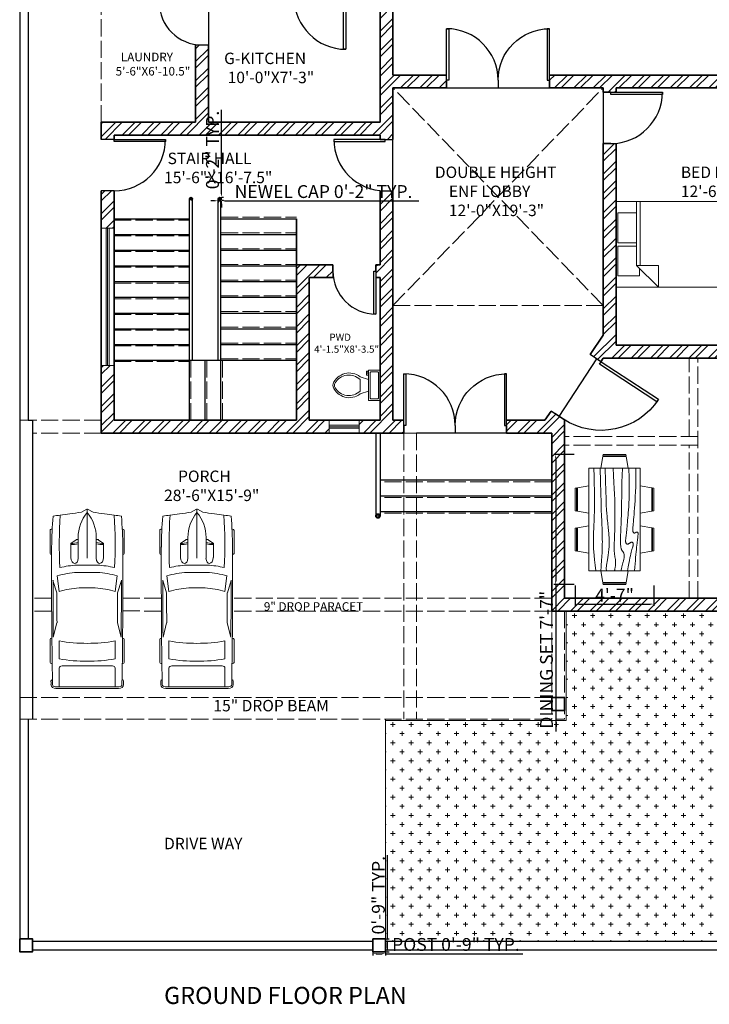
# Model space of a CAD drawing. Units: inches. Extents: x 839 to 1638, y 2998 to 4342.
# Tile 1 of 4: x 839 to 1321, y 3024 to 3713. Entities that reach past the tile are written whole.
import ezdxf

# ---------------------------------------------------------------- set-up
doc = ezdxf.new("R2010")
doc.units = ezdxf.units.IN
doc.linetypes.add('ACAD_ISO02W100', pattern=[15, 12, -3])
for name, color, linetype, lineweight in [('A-ANNO-DIMS', 2, 'Continuous', 18), ('A-ANNO-TEXT', 7, 'Continuous', 18), ('A-ANNO-TITL', 7, 'Continuous', 30), ('A-AREA-IDEN', 7, 'Continuous', 18), ('A-COLS', 7, 'Continuous', 35), ('A-DOOR', 4, 'Continuous', 25), ('A-DOOR-JAMB', 7, 'Continuous', 25), ('A-FLOR-FIXT', 9, 'Continuous', 18), ('A-FLOR-OVHD', 8, 'ACAD_ISO02W100', 18), ('A-FLOR-STRS', 7, 'Continuous', 25), ('A-FLOR-STRS-HIDN', 8, 'ACAD_ISO02W100', 13), ('A-FURN', 8, 'Continuous', 18), ('A-WALL', 7, 'Continuous', 35), ('A-WALL-OVHD', 8, 'ACAD_ISO02W100', 18), ('A-WALL-PATT', 252, 'Continuous', 13), ('C-PROP', 7, 'Continuous', 30), ('C-SITE-VEHS', 8, 'Continuous', 13), ('L-HRDS', 8, 'Continuous', 18)]:
    doc.layers.add(name, color=color, linetype=linetype, lineweight=lineweight)
doc.layers.add('A-GLAZ', color=244, linetype='Continuous', lineweight=20, true_color=0x991b1e)
doc.layers.add('L-SITE-PATT', color=116, linetype='Continuous', lineweight=13, true_color=0x136734)
doc.styles.get("Standard").update_dxf_attribs({"font": 'arial.ttf'})
doc.dimstyles.new('ISO-25', dxfattribs={"dimtxt": 9, "dimasz": 2.5, "dimexe": 1.25, "dimexo": 0.625, "dimtad": 1, "dimlunit": 3, "dimtxsty": 'Standard', "dimcen": 2.5, "dimadec": 0, "dimazin": 0, "dimtfac": 1, "dimtmove": 0, "dimatfit": 3, "dimfxl": 1, "dimarcsym": 0})

# ---------------------------------------------------------------- blocks, each defined once
blk = doc.blocks.new('*U3')
for p, q in [((-40, 0), (-40, 6)), ((0, 0), (0, 6))]:
    blk.add_line(p, q)
blk.add_lwpolyline([(0, 0), (0, -40), (-1.75, -40), (-1.75, 0)], close=True)
blk.add_arc((0, 0), 40, 180, 270)
blk = doc.blocks.new('*U2')
for p, q in [((0, 0), (0, -6)), ((40, 0), (40, -6))]:
    blk.add_line(p, q)
blk.add_lwpolyline([(0, 0), (0, 40), (1.75, 40), (1.75, 0)], close=True)
blk.add_arc((0, 0), 40, 0, 90)
blk = doc.blocks.new('*U6')
for p, q in [((0, 0), (0, -6)), ((-40, 0), (-40, -6))]:
    blk.add_line(p, q)
blk.add_lwpolyline([(0, 0), (0, 40), (-1.75, 40), (-1.75, 0)], close=True)
blk.add_arc((0, 0), 40, 90, 180)
blk = doc.blocks.new('*U7')
for p, q in [((-40, 0), (-40, 6)), ((0, 0), (0, 6))]:
    blk.add_line(p, q)
blk.add_lwpolyline([(0, 0), (0, -40), (-1.75, -40), (-1.75, 0)], close=True)
blk.add_arc((0, 0), 40, 180, 270)
blk = doc.blocks.new('*U10')
for p, q in [((0, 0), (0, 6)), ((40, 0), (40, 6))]:
    blk.add_line(p, q)
blk.add_lwpolyline([(0, 0), (0, -40), (1.75, -40), (1.75, 0)], close=True)
blk.add_arc((0, 0), 40, 270, 360)
blk = doc.blocks.new('*U11')
for p, q in [((0, 0), (0, -6)), ((-40, 0), (-40, -6))]:
    blk.add_line(p, q)
blk.add_lwpolyline([(0, 0), (0, 40), (-1.75, 40), (-1.75, 0)], close=True)
blk.add_arc((0, 0), 40, 90, 180)
blk = doc.blocks.new('*U12')
for p, q in [((-40, 0), (-40, 6)), ((0, 0), (0, 6))]:
    blk.add_line(p, q)
blk.add_lwpolyline([(0, 0), (0, -40), (-1.75, -40), (-1.75, 0)], close=True)
blk.add_arc((0, 0), 40, 180, 270)
blk = doc.blocks.new('*U15')
for p, q in [((9.5, -6), (9.5, -2)), ((-10, -8.5), (-8, -8.5)), ((-10, -9.5), (-10, -8.5)), ((-7, -9.5), (-10, -9.5)), ((-8, -8.5), (-8, -8)), ((-7, -8), (-7, -9.5)), ((-4, -8), (-6, -14)), ((4, -8), (6, -14)), ((4, -14), (-4, -14))]:
    blk.add_line(p, q)
blk.add_lwpolyline([(10.5, -8), (10.5, 0), (-10.5, 0), (-10.5, -8)], close=True)
for points in [[(-9.5, -2), (-9.5, -6)], [(8.5, -1), (-8.5, -1)], [(-8.5, -7), (8.5, -7)]]:
    blk.add_lwpolyline(points)
for centre, radius, start, end in [((-8.62, -1.88), 0.884, 81.8699, 188.1301), ((-8.62, -6.12), 0.884, 171.8699, 278.1301), ((8.62, -1.88), 0.884, 351.8699, 98.1301), ((8.62, -6.12), 0.884, 261.8699, 8.1301), ((3.52, -21.58), 12.17, 141.46911, 247.97143), ((4.2, -21.82), 11.33, 136.36773, 238.94682), ((-3.52, -21.58), 12.17, 292.02843, 38.53071), ((-4.2, -21.82), 11.33, 301.05301, 43.63209), ((0, -27.88), 4, 245.73182, 294.26817), ((0, -29), 4, 254.86053, 285.13947)]:
    blk.add_arc(centre, radius, start, end)
blk = doc.blocks.new('Bed - Queen')
for p, q in [((0, -80.00003), (0, 0)), ((0, 0), (59.99999, 0)), ((59.99999, 0), (59.99999, -80.00003)), ((7.99999, -1.2), (28.79998, -1.2)), ((7.99999, -14.4), (7.99999, -1.2)), ((28.79998, -1.2), (28.79998, -14.4)), ((31.19999, -1.2), (51.99999, -1.2)), ((31.19999, -14.4), (31.19999, -1.2)), ((51.99999, -1.2), (51.99999, -16.4)), ((0, -14.4), (44.8, -14.4)), ((44.8, -16.8), (0, -16.8)), ((59.99999, -29.6), (44.8, -14.4)), ((44.8, -14.4), (44.8, -29.6)), ((51.99999, -16.4), (46.79936, -16.4)), ((44.8, -29.6), (59.99999, -29.6)), ((59.99999, -80.00003), (0, -80.00003))]:
    blk.add_line(p, q)
blk = doc.blocks.new('Dining Set - 36 x 72 in.')
for p, q in [((-22.2343, 26.00059), (-23.4847, 17.99762)), ((-22.2304, 26), (-5.7608, 26)), ((-22, 27.5), (-22.1562, 26.50042)), ((-5.8416, 26.5), (-22.1534, 26.5)), ((-22, 27.5), (-6, 27.5)), ((-5.8437, 26.49966), (-6, 27.5)), ((-4.5152, 17.99762), (-5.7655, 25.99926)), ((5.7657, 26.00059), (4.5153, 17.99762)), ((5.7696, 26), (22.2392, 26)), ((6, 27.5), (5.8438, 26.50042)), ((22.1584, 26.5), (5.8466, 26.5)), ((6, 27.5), (22, 27.5)), ((22.1563, 26.49966), (22, 27.5)), ((23.4848, 17.99762), (22.2345, 25.99926)), ((36, 18), (-36, 18)), ((-36, 18), (-36, -18)), ((36, -18), (36, 18)), ((-45.5, 8), (-44.5004, 8.15617)), ((-45.5, 8), (-45.5, -8)), ((-44.5, -8.15843), (-44.5, 8.15338)), ((-44.0006, 8.23428), (-35.9976, 9.48474)), ((-44, 8.23041), (-44, -8.23915)), ((44.0006, 8.23428), (35.9976, 9.48474)), ((44, 8.23041), (44, -8.23915)), ((44.5, -8.15843), (44.5, 8.15338)), ((45.5, 8), (44.5005, 8.15617)), ((45.5, 8), (45.5, -8)), ((-44.4997, -8.15631), (-45.5, -8)), ((-35.9976, -9.48476), (-43.9993, -8.2345)), ((35.9976, -9.48476), (43.9993, -8.2345)), ((44.4997, -8.15631), (45.5, -8)), ((-36, -18), (36, -18)), ((-22.2343, -26.0006), (-23.4847, -17.99762)), ((-4.5152, -17.99762), (-5.7655, -25.99928)), ((5.7657, -26.0006), (4.5153, -17.99762)), ((23.4848, -17.99762), (22.2345, -25.99928)), ((-22.2304, -26), (-5.7608, -26)), ((-22, -27.5), (-22.1562, -26.50044)), ((-5.8416, -26.5), (-22.1534, -26.5)), ((-22, -27.5), (-6, -27.5)), ((-5.8437, -26.49967), (-6, -27.5)), ((5.7696, -26), (22.2392, -26)), ((6, -27.5), (5.8438, -26.50044)), ((22.1584, -26.5), (5.8466, -26.5)), ((6, -27.5), (22, -27.5)), ((22.1563, -26.49967), (22, -27.5))]:
    blk.add_line(p, q)
for points in [[(-36, 15), (-31.1772, 14.97754), (-26.8079, 14.91406), (-22.8538, 14.81543), (-19.276, 14.6875), (-16.0362, 14.53613), (-13.0957, 14.36718), (-10.4159, 14.18652), (-7.9583, 14), (-5.6904, 13.81315), (-3.6035, 13.63021), (-1.6954, 13.45508), (0.0365, 13.29166), (1.5945, 13.14388), (2.9811, 13.01562), (4.1988, 12.9108), (5.25, 12.83333), (6.1393, 12.78613), (6.8802, 12.76823), (7.4883, 12.77767), (7.9792, 12.8125), (8.3685, 12.87077), (8.6719, 12.95052), (8.9049, 13.0498), (9.0833, 13.16666), (9.2205, 13.29899), (9.3216, 13.44401), (9.3895, 13.59879), (9.4271, 13.76041), (9.4373, 13.92594), (9.4232, 14.09245), (9.3875, 14.257), (9.3333, 14.41666), (9.2638, 14.56917), (9.1836, 14.71484), (9.0975, 14.85465), (9.0104, 14.98958), (8.9272, 15.1206), (8.8529, 15.2487), (8.7922, 15.37483), (8.75, 15.5), (8.7305, 15.62467), (8.7344, 15.74739), (8.7617, 15.86621), (8.8125, 15.97916), (8.8867, 16.08431), (8.9844, 16.17968), (9.1055, 16.26334), (9.25, 16.33333), (9.4189, 16.38802), (9.6172, 16.42708), (9.8506, 16.45052), (10.125, 16.45833), (10.4463, 16.45052), (10.8203, 16.42708), (11.2529, 16.38802), (11.75, 16.33333), (12.3184, 16.26318), (12.9694, 16.17838), (13.7151, 16.07991), (14.5677, 15.96875), (15.5395, 15.84586), (16.6426, 15.71224), (17.8893, 15.56884), (19.2917, 15.41666), (20.859, 15.25667), (22.5879, 15.08984), (24.4721, 14.91715), (26.5052, 14.73958), (28.6809, 14.5581), (30.9929, 14.3737), (33.4347, 14.18733), (36, 14)], [(-36, 10), (-28.9766, 10.14274), (-23.1725, 10.20442), (-18.4241, 10.19775), (-14.5677, 10.13541), (-11.4399, 10.03011), (-8.877, 9.89453), (-6.7154, 9.74137), (-4.7917, 9.58333), (-2.9698, 9.43082), (-1.2246, 9.28515), (0.4415, 9.14534), (2.026, 9.01041), (3.5266, 8.87939), (4.9408, 8.7513), (6.266, 8.62516), (7.5, 8.5), (8.6411, 8.37549), (9.6914, 8.2539), (10.6538, 8.13818), (11.5312, 8.03125), (12.3267, 7.93603), (13.043, 7.85547), (13.6831, 7.79248), (14.25, 7.75), (14.7471, 7.7303), (15.1797, 7.73307), (15.5537, 7.75732), (15.875, 7.80208), (16.1494, 7.86637), (16.3828, 7.94922), (16.5811, 8.04964), (16.75, 8.16666), (16.8944, 8.29915), (17.0143, 8.44531), (17.1089, 8.60319), (17.1771, 8.77083), (17.218, 8.94629), (17.2305, 9.1276), (17.2137, 9.31282), (17.1667, 9.5), (17.0895, 9.6875), (16.987, 9.875), (16.8649, 10.0625), (16.7292, 10.25), (16.5856, 10.4375), (16.4401, 10.625), (16.2985, 10.8125), (16.1667, 11), (16.05, 11.18733), (15.9518, 11.3737), (15.8752, 11.5581), (15.8229, 11.73958), (15.798, 11.91715), (15.8034, 12.08984), (15.842, 12.25667), (15.9167, 12.41666), (16.0295, 12.56836), (16.1784, 12.70833), (16.3605, 12.83268), (16.5729, 12.9375), (16.8127, 13.01888), (17.0768, 13.07291), (17.3625, 13.0957), (17.6667, 13.08333), (17.9894, 13.03312), (18.3418, 12.94726), (18.7382, 12.82918), (19.1927, 12.68229), (19.7195, 12.51001), (20.3327, 12.31575), (21.0465, 12.10294), (21.875, 11.875), (22.8357, 11.63354), (23.959, 11.37304), (25.2786, 11.08618), (26.8282, 10.76562), (28.6414, 10.40405), (30.752, 9.99414), (33.1936, 9.52856), (36, 9)], [(-36, 5.5), (-30.7157, 5.3348), (-26.069, 5.20963), (-21.9946, 5.11767), (-18.4271, 5.05208), (-15.3009, 5.00602), (-12.5508, 4.97265), (-10.1112, 4.94515), (-7.9167, 4.91666), (-5.909, 4.88167), (-4.0586, 4.83984), (-2.3429, 4.79215), (-0.7396, 4.73958), (0.7739, 4.6831), (2.22, 4.6237), (3.6213, 4.56233), (5, 4.5), (6.373, 4.43782), (7.7344, 4.3776), (9.0723, 4.32129), (10.375, 4.27083), (11.6309, 4.22819), (12.8281, 4.19531), (13.9551, 4.17415), (15, 4.16666), (15.954, 4.17448), (16.819, 4.19791), (17.6001, 4.23698), (18.3021, 4.29166), (18.9299, 4.36198), (19.4883, 4.44791), (19.9823, 4.54948), (20.4167, 4.66666), (20.7969, 4.79899), (21.1302, 4.94401), (21.4245, 5.09879), (21.6875, 5.26041), (21.9271, 5.42594), (22.1511, 5.59245), (22.3672, 5.757), (22.5834, 5.91666), (22.8065, 6.06868), (23.0404, 6.21093), (23.2879, 6.34147), (23.5521, 6.45833), (23.8358, 6.55957), (24.142, 6.64323), (24.4735, 6.70735), (24.8334, 6.75), (25.2235, 6.76969), (25.642, 6.76692), (26.0858, 6.74267), (26.5521, 6.69791), (27.0379, 6.63362), (27.5404, 6.55078), (28.0565, 6.45036), (28.5834, 6.33333), (29.1242, 6.19987), (29.7071, 6.04687), (30.3661, 5.87044), (31.1354, 5.66666), (32.0493, 5.43164), (33.142, 5.16146), (34.4475, 4.85221), (36, 4.5)], [(-36, -1), (-30.7915, -0.6591), (-26.0195, -0.38216), (-21.6519, -0.16284), (-17.6563, 0.00521), (-14.0005, 0.12833), (-10.6523, 0.21289), (-7.5796, 0.26522), (-4.75, 0.29166), (-2.134, 0.29793), (0.2878, 0.28711), (2.5317, 0.26163), (4.6146, 0.22396), (6.5529, 0.17651), (8.3633, 0.12174), (10.0623, 0.06209), (11.6667, 0), (13.1899, -0.06201), (14.6341, -0.1211), (15.9982, -0.17432), (17.2813, -0.21875), (18.4823, -0.25147), (19.6003, -0.26953), (20.6343, -0.27002), (21.5834, -0.25), (22.4481, -0.20768), (23.2357, -0.14584), (23.9549, -0.06836), (24.6146, 0.02083), (25.2235, 0.11784), (25.7904, 0.21875), (26.3241, 0.31966), (26.8334, 0.41666), (27.3265, 0.50618), (27.8099, 0.58593), (28.2894, 0.65397), (28.7709, 0.70833), (29.2601, 0.74707), (29.763, 0.76823), (30.2855, 0.76985), (30.8334, 0.75), (31.4088, 0.70784), (31.9994, 0.64713), (32.589, 0.57275), (33.1615, 0.48958), (33.7008, 0.4025), (34.1908, 0.3164), (34.6153, 0.23616), (34.9584, 0.16666), (35.2099, 0.11165), (35.3848, 0.07031), (35.504, 0.04069), (35.5886, 0.02083), (35.6594, 0.00879), (35.7377, 0.0026), (35.8442, 0.00032), (36, 0)], [(-36, -6.5), (-27.1843, -6.31267), (-20.084, -6.1263), (-14.469, -5.9419), (-10.1094, -5.76042), (-6.7752, -5.58285), (-4.2363, -5.41016), (-2.2629, -5.24333), (-0.625, -5.08334), (0.8708, -4.93099), (2.2715, -4.78646), (3.5872, -4.64974), (4.8281, -4.52084), (6.0046, -4.39974), (7.127, -4.28646), (8.2053, -4.18099), (9.25, -4.08334), (10.2705, -3.99382), (11.2734, -3.91407), (12.2647, -3.84603), (13.25, -3.79167), (14.2354, -3.75293), (15.2266, -3.73177), (16.2295, -3.73015), (17.25, -3.75), (18.2912, -3.79248), (19.3451, -3.85547), (20.4009, -3.93604), (21.4479, -4.03125), (22.4754, -4.13819), (23.4727, -4.25391), (24.4289, -4.37549), (25.3334, -4.5), (26.1785, -4.62492), (26.9694, -4.74935), (27.7145, -4.87281), (28.4219, -4.99479), (29.1, -5.11483), (29.7572, -5.23242), (30.4016, -5.34709), (31.0417, -5.45834), (31.6837, -5.56437), (32.3262, -5.65821), (32.9658, -5.73153), (33.599, -5.77604), (34.2224, -5.78345), (34.8327, -5.74545), (35.4264, -5.65373), (36, -5.5)], [(-36, -10), (-26.4022, -9.81299), (-18.4675, -9.62891), (-11.9839, -9.45069), (-6.7396, -9.28125), (-2.5226, -9.12354), (0.8789, -8.98047), (3.6769, -8.85498), (6.0833, -8.75), (8.2767, -8.66765), (10.3021, -8.60677), (12.1712, -8.56543), (13.8958, -8.54167), (15.4876, -8.53353), (16.9583, -8.53907), (18.3197, -8.55632), (19.5834, -8.58334), (20.7616, -8.61841), (21.8685, -8.66081), (22.9188, -8.71004), (23.9271, -8.76563), (24.9081, -8.82707), (25.8763, -8.89388), (26.8465, -8.96558), (27.8334, -9.04167), (28.8474, -9.12118), (29.8828, -9.20117), (30.93, -9.27824), (31.9792, -9.34896), (33.0205, -9.40991), (34.0443, -9.45768), (35.0407, -9.48885), (36, -9.5)], [(-36, -14.5), (-30.0881, -14.33513), (-25.0332, -14.21224), (-20.7312, -14.12647), (-17.0781, -14.07292), (-13.97, -14.04671), (-11.3027, -14.04297), (-8.9724, -14.05681), (-6.875, -14.08334), (-4.9224, -14.11833), (-3.0905, -14.16016), (-1.3709, -14.20785), (0.2448, -14.26042), (1.7647, -14.3169), (3.1973, -14.3763), (4.5507, -14.43767), (5.8333, -14.5), (7.0554, -14.5621), (8.235, -14.62175), (9.3922, -14.67652), (10.5469, -14.72396), (11.7192, -14.76164), (12.929, -14.78711), (14.1965, -14.79794), (15.5417, -14.79167), (16.9933, -14.76424), (18.6152, -14.70508), (20.4804, -14.60197), (22.6615, -14.44271), (25.2312, -14.21509), (28.2624, -13.9069), (31.8277, -13.50594), (36, -13)]]:
    blk.add_lwpolyline(points)
blk = doc.blocks.new('*U19')
for p, q in [((21.1, 37.4), (21.1, 36.8)), ((46.6, 38.9), (22.4, 38.9)), ((47.8, 37.4), (47.8, 37.4)), ((70, 31.5), (86.4, 29.4)), ((88, 31.9), (74.8, 35.9)), ((134.3, 35.6), (119.3, 31.8)), ((135.5, 37.1), (135.5, 37.4)), ((136.7, 38.9), (160.9, 38.9)), ((162.1, 37.4), (162.1, 36.8)), ((186.5, -33.5), (186.5, 33.5)), ((188.4, -32.8), (188.4, 32.8)), ((138.4, 29.4), (157.2, 29.4)), ((164.5, 26.4), (164.5, -26.4)), ((186.5, 29.4), (167, 29.4)), ((32.1, 9.5), (32.1, 11.2)), ((32.3, 11.6), (36.1, 17.2)), ((36.1, 17.2), (50.9, 17.2)), ((58.9, -10.8), (58.9, 10.8)), ((66.6, -10.5), (66.6, 10.5)), ((186.5, -10.5), (186.5, 10.5)), ((3.3, 6.1), (0.1, 0.4)), ((29.8, 9.5), (51.7, 9.5)), ((82.7, 8.5), (82.7, -8.5)), ((0, 0), (51.7, 0)), ((0.1, -0.4), (3.3, -6.1)), ((29.8, -9.5), (51.7, -9.5)), ((32.1, -9.5), (32.1, -11.2)), ((32.3, -11.6), (36.1, -17.2)), ((36.1, -17.2), (50.9, -17.2)), ((86.4, -29.4), (70, -31.5)), ((157.2, -29.4), (138.4, -29.4)), ((167, -29.4), (186.5, -29.4)), ((21.1, -37.4), (21.1, -36.8)), ((46.6, -38.9), (22.4, -38.9)), ((47.8, -37.4), (47.8, -37.4)), ((88, -31.9), (74.8, -35.9)), ((134.3, -35.6), (119.3, -31.8)), ((135.5, -37.1), (135.5, -37.4)), ((136.7, -38.9), (160.9, -38.9)), ((162.1, -37.4), (162.1, -36.8))]:
    blk.add_line(p, q)
for centre, major_axis, ratio, start_param, end_param in [((266, -27.5), (0, 313.3), 0.842304, 1.367076, 1.39176), ((41.2, -490.9), (0, 528.2), 0.842304, 0.00281, 0.075598), ((22.4, 37.4), (0, -1.48), 0.842304, 3.141593, 4.712389), ((64.5, -10555.6), (0, 10593), 0.842304, -0.013397, 0.002797), ((46.6, 37.4), (0, 1.48), 0.842304, -1.570796, 0), ((135.3, 5.4), (0, 81.8), 0.842304, 1.245306, 1.50788), ((64.5, -10555.6), (0, -10591.5), 0.842304, 3.133765, 3.140441), ((95.8, -3666.4), (0, -3698.2), 0.842304, 3.134049, 3.144098), ((136.7, 37.4), (0, -1.48), 0.842304, 3.141593, 4.712389), ((160.9, 37.4), (0, 1.48), 0.842304, -1.570796, 0), ((180.6, 35.8), (0, 2.22), 0.842304, -0.013017, 1.249894), ((64.5, -10556.4), (0, 10595.3), 0.842304, -0.013397, -0.013017), ((184, 32.8), (0, -5.25), 0.842304, 1.570796, 3.128196), ((184, 33.5), (0, -2.96), 0.842304, 1.570796, 3.128196), ((259.2, -27.5), (0, -305.3), 0.842304, 4.528606, 4.561838), ((37.5, -594), (0, -623.3), 0.842304, 3.096046, 3.200911), ((134.4, 5.4), (0, -89.8), 0.842304, 4.449482, 4.652344), ((149.6, 2.8), (0, -79.6), 0.842304, 4.372215, 4.640744), ((17.1, 0), (0, 147), 0.842304, 4.511394, 4.913384), ((35.9, 0), (0, 147), 0.842304, 4.511394, 4.913384), ((167, 26.4), (0, 2.96), 0.842304, 0, 1.570796), ((-204.5, 52.4), (0, -251), 0.842304, 1.385369, 1.434372), ((32.7, 11.2), (0, 0.74), 0.842304, 0.879714, 1.570796), ((13, 17), (0, 27.4), 0.842304, 4.435146, 4.718221), ((14.2, 17), (0, 27.4), 0.842304, 4.435146, 4.718221), ((50.8, 13.3), (6.34, -0.36), 0.603834, -1.395552, 1.581315), ((0.6, 0), (0, -0.74), 0.842304, 4.131459, 5.293319), ((29.8, -46.7), (0, 56.2), 0.842304, 0, 0.590319), ((-204.5, -52.4), (0, 251), 0.842304, -1.434372, -1.385369), ((29.8, 46.7), (0, 56.2), 0.842304, 2.551274, 3.141593), ((13, -17), (0, -27.4), 0.842304, 1.564964, 1.848039), ((14.2, -17), (0, -27.4), 0.842304, 1.564964, 1.848039), ((149.6, -2.8), (0, -79.6), 0.842304, -1.499151, -1.230623), ((259.2, 27.5), (0, 305.3), 0.842304, 1.721348, 1.754579), ((32.7, -11.2), (0, -0.74), 0.842304, 4.712389, 5.403472), ((134.4, -5.4), (0, -89.8), 0.842304, -1.510751, -1.307889), ((135.3, -5.4), (0, -81.8), 0.842304, -1.50788, -1.245306), ((266, 27.5), (0, 313.3), 0.842304, 1.749832, 1.774517), ((37.5, 594), (0, -623.3), 0.842304, -0.059319, 0.045547), ((167, -26.4), (0, -2.96), 0.842304, 4.712389, 6.283185), ((41.2, 490.9), (0, -528.2), 0.842304, -0.075598, -0.00281), ((22.4, -37.4), (0, 1.48), 0.842304, 1.570796, 3.141593), ((64.5, 10555.6), (0, 10593), 0.842304, 3.138796, 3.15499), ((46.6, -37.4), (0, -1.48), 0.842304, 0, 1.570796), ((64.5, 10555.6), (0, -10591.5), 0.842304, 0.001152, 0.007828), ((95.8, 3666.4), (0, -3698.2), 0.842304, -0.002505, 0.007544), ((136.7, -37.4), (0, -1.48), 0.842304, -1.570796, 0), ((160.9, -37.4), (0, 1.48), 0.842304, 3.141593, 4.712389), ((180.6, -35.8), (0, -2.22), 0.842304, -1.249894, 0.013017), ((64.5, 10556.4), (0, 10595.3), 0.842304, 3.15461, 3.15499), ((184, -32.8), (0, -5.25), 0.842304, 0.013397, 1.570796), ((184, -33.5), (0, 2.96), 0.842304, 3.15499, 4.712389)]:
    blk.add_ellipse(centre, major_axis=major_axis, ratio=ratio, start_param=start_param, end_param=end_param)
at = {"extrusion": (0, 0, -1)}
blk.add_ellipse((50.8, -13.3), major_axis=(6.34, 0.36), ratio=0.603834, start_param=-1.395552, end_param=1.581315, dxfattribs=at)
blk = doc.blocks.new('WIN-21x9')
for p, q in [((0, 5.5), (21, 5.5)), ((0, 4.5), (21, 4.5)), ((0, 3.5), (21, 3.5))]:
    blk.add_line(p, q)
blk.add_lwpolyline([(0, 9), (21, 9), (21, 0), (0, 0)], close=True)
blk = doc.blocks.new('POST-9x9')
blk.add_lwpolyline([(0, 9), (9, 9), (9, 0), (0, 0)], close=True)
blk = doc.blocks.new('RAIL-NEWEL-CAP')
for radius in [1.07, 0.767, 0.467]:
    blk.add_circle((1.07, 1.07), radius)
blk = doc.blocks.new('*D30')
at = {"layer": 'A-ANNO-DIMS', "color": 0, "lineweight": -2, "transparency": 16777216}
for p, q in [((1086, 3059.91), (1086, 3057.94)), ((1088.5, 3059.19), (1092.5, 3059.19)), ((1095, 3059.91), (1095, 3057.94)), ((1095, 3059.19), (1190.88, 3059.19))]:
    blk.add_line(p, q, dxfattribs=at)
at = {"layer": 'A-ANNO-DIMS', "color": 0, "transparency": 16777216}
for points in [[(1088.5, 3059.6), (1088.5, 3058.77), (1086, 3059.19)], [(1092.5, 3059.6), (1092.5, 3058.77), (1095, 3059.19)]]:
    blk.add_solid(points, dxfattribs=at)
at = {"layer": 'Defpoints', "color": 0, "transparency": 16777216}
for p in [(1086, 3060.54), (1095, 3060.54), (1095, 3059.19)]:
    blk.add_point(p, dxfattribs=at)
at = {"layer": 'A-ANNO-DIMS', "color": 0, "transparency": 16777216, "insert": (1144.19, 3064.47), "char_height": 9, "attachment_point": 5}
blk.add_mtext('POST 0\'-9" TYP.', dxfattribs=at)
blk = doc.blocks.new('*D31')
at = {"layer": 'A-ANNO-DIMS', "color": 0, "lineweight": -2, "transparency": 16777216}
for p, q in [((1096.35, 3069.54), (1096.35, 3128.15)), ((1095.62, 3069.54), (1097.6, 3069.54)), ((1096.35, 3063.04), (1096.35, 3067.04)), ((1095.62, 3060.54), (1097.6, 3060.54))]:
    blk.add_line(p, q, dxfattribs=at)
at = {"layer": 'A-ANNO-DIMS', "color": 0, "transparency": 16777216}
for points in [[(1095.93, 3067.04), (1096.76, 3067.04), (1096.35, 3069.54)], [(1095.93, 3063.04), (1096.76, 3063.04), (1096.35, 3060.54)]]:
    blk.add_solid(points, dxfattribs=at)
at = {"layer": 'Defpoints', "color": 0, "transparency": 16777216}
for p in [(1095, 3069.54), (1096.35, 3069.54), (1095, 3060.54)]:
    blk.add_point(p, dxfattribs=at)
at = {"layer": 'A-ANNO-DIMS', "color": 0, "transparency": 16777216, "insert": (1091.13, 3100.09), "char_height": 9, "attachment_point": 5, "rotation": 90}
blk.add_mtext('0\'-9" TYP.', dxfattribs=at)
blk = doc.blocks.new('*D46')
at = {"layer": 'A-ANNO-DIMS', "color": 0, "lineweight": -2, "transparency": 16777216}
for p, q in [((975.39, 3585.87), (972.89, 3585.87)), ((977.89, 3585.87), (980.02, 3585.87)), ((977.89, 3585.57), (977.89, 3584.62)), ((980.02, 3585.57), (980.02, 3584.62)), ((982.52, 3585.87), (1118.25, 3585.87))]:
    blk.add_line(p, q, dxfattribs=at)
at = {"layer": 'A-ANNO-DIMS', "color": 0, "transparency": 16777216}
for points in [[(975.39, 3586.29), (975.39, 3585.46), (977.89, 3585.87)], [(982.52, 3586.29), (982.52, 3585.46), (980.02, 3585.87)]]:
    blk.add_solid(points, dxfattribs=at)
at = {"layer": 'Defpoints', "color": 0, "transparency": 16777216}
for p in [(977.89, 3586.19), (980.02, 3586.19), (980.02, 3585.87)]:
    blk.add_point(p, dxfattribs=at)
at = {"layer": 'A-ANNO-DIMS', "color": 0, "transparency": 16777216, "insert": (1051.63, 3591.15), "char_height": 9, "attachment_point": 5}
blk.add_mtext('NEWEL CAP 0\'-2" TYP.', dxfattribs=at)
blk = doc.blocks.new('*D47')
at = {"layer": 'A-ANNO-DIMS', "color": 0, "lineweight": -2, "transparency": 16777216}
for p, q in [((980.34, 3590.83), (980.34, 3649.44)), ((980.34, 3586.19), (980.34, 3588.33)), ((980.34, 3583.69), (980.34, 3581.19)), ((980.65, 3588.33), (981.59, 3588.33)), ((980.65, 3586.19), (981.59, 3586.19))]:
    blk.add_line(p, q, dxfattribs=at)
at = {"layer": 'A-ANNO-DIMS', "color": 0, "transparency": 16777216}
for points in [[(979.93, 3590.83), (980.76, 3590.83), (980.34, 3588.33)], [(979.93, 3583.69), (980.76, 3583.69), (980.34, 3586.19)]]:
    blk.add_solid(points, dxfattribs=at)
at = {"layer": 'Defpoints', "color": 0, "transparency": 16777216}
for p in [(980.02, 3588.33), (980.02, 3586.19), (980.34, 3588.33)]:
    blk.add_point(p, dxfattribs=at)
at = {"layer": 'A-ANNO-DIMS', "color": 0, "transparency": 16777216, "insert": (975.12, 3621.38), "char_height": 9, "attachment_point": 5, "rotation": 90}
blk.add_mtext('0\'-2" TYP.', dxfattribs=at)
blk = doc.blocks.new('*D48')
at = {"layer": 'A-ANNO-DIMS', "color": 0, "lineweight": -2, "transparency": 16777216}
for p, q in [((1226.99, 3408.39), (1212.71, 3408.39)), ((1213.96, 3405.89), (1213.96, 3319.89)), ((1226.99, 3317.39), (1212.71, 3317.39)), ((1213.96, 3317.39), (1213.96, 3214.72))]:
    blk.add_line(p, q, dxfattribs=at)
at = {"layer": 'A-ANNO-DIMS', "color": 0, "transparency": 16777216}
for points in [[(1213.54, 3405.89), (1214.38, 3405.89), (1213.96, 3408.39)], [(1213.54, 3319.89), (1214.38, 3319.89), (1213.96, 3317.39)]]:
    blk.add_solid(points, dxfattribs=at)
at = {"layer": 'Defpoints', "color": 0, "transparency": 16777216}
for p in [(1227.61, 3408.39), (1213.96, 3317.39), (1227.61, 3317.39)]:
    blk.add_point(p, dxfattribs=at)
at = {"layer": 'A-ANNO-DIMS', "color": 0, "transparency": 16777216, "insert": (1208.68, 3264.81), "char_height": 9, "attachment_point": 5, "rotation": 90}
blk.add_mtext('DINING SET 7\'-7"', dxfattribs=at)
blk = doc.blocks.new('*D49')
at = {"layer": 'A-ANNO-DIMS', "color": 0, "lineweight": -2, "transparency": 16777216}
for p, q in [((1227.61, 3316.77), (1227.61, 3302.49)), ((1282.61, 3316.77), (1282.61, 3302.49)), ((1230.11, 3303.74), (1280.11, 3303.74))]:
    blk.add_line(p, q, dxfattribs=at)
at = {"layer": 'A-ANNO-DIMS', "color": 0, "transparency": 16777216}
for points in [[(1230.11, 3304.16), (1230.11, 3303.32), (1227.61, 3303.74)], [(1280.11, 3304.16), (1280.11, 3303.32), (1282.61, 3303.74)]]:
    blk.add_solid(points, dxfattribs=at)
at = {"layer": 'Defpoints', "color": 0, "transparency": 16777216}
for p in [(1227.61, 3317.39), (1282.61, 3317.39), (1282.61, 3303.74)]:
    blk.add_point(p, dxfattribs=at)
at = {"layer": 'A-ANNO-DIMS', "color": 0, "transparency": 16777216, "insert": (1255.11, 3308.87), "char_height": 9, "attachment_point": 5}
blk.add_mtext('4\'-7"', dxfattribs=at)

msp = doc.modelspace()

# ---------------------------------------------------------------- hatches: boundary and pattern name
at = {"layer": 'A-WALL-PATT'}
h = msp.add_hatch(dxfattribs=at)
h.set_pattern_fill('ANSI32', color=256)
h.paths.add_polyline_path([(1440.674, 3673.836), (1430.169, 3673.836), (1430.169, 3724.836), (1421.169, 3724.836), (1421.169, 3673.836), (1209.669, 3673.836), (1209.669, 3670.236), (1209.669, 3664.836), (1247.169, 3664.836), (1247.169, 3661.836), (1252.569, 3661.836), (1256.169, 3661.836), (1256.169, 3664.836), (1440.674, 3664.836)])
h.paths.add_polyline_path([(1137.669, 3673.836), (1100.169, 3673.836), (1100.169, 3733.836), (1091.169, 3733.836), (1067.169, 3733.836), (1067.169, 3727.836), (1091.169, 3727.836), (1091.169, 3640.836), (971.169, 3640.836), (971.169, 3694.836), (962.169, 3694.836), (962.169, 3640.836), (896.169, 3640.836), (896.169, 3628.836), (905.169, 3628.836), (905.169, 3631.836), (1091.169, 3631.836), (1091.169, 3628.836), (1100.169, 3628.836), (1100.169, 3664.836), (1137.669, 3664.836)])
h.paths.add_polyline_path([(1256.169, 3625.836), (1247.169, 3625.836), (1247.169, 3491.75), (1237.967, 3478.332), (1245.508, 3473.161), (1247.169, 3475.836), (1520.169, 3475.836), (1520.169, 3595.836), (1504.368, 3595.836), (1504.368, 3586.836), (1511.169, 3586.836), (1511.169, 3484.836), (1439.169, 3484.836), (1439.169, 3550.955), (1415.169, 3550.955), (1415.169, 3586.836), (1418.169, 3586.836), (1418.169, 3595.836), (1406.169, 3595.836), (1406.169, 3544.955), (1433.169, 3544.955), (1433.169, 3484.836), (1406.169, 3484.836), (1256.169, 3484.836)])
h.paths.add_polyline_path([(1483.368, 3595.836), (1472.169, 3595.836), (1472.169, 3600.336), (1463.169, 3600.336), (1463.169, 3595.836), (1448.169, 3595.836), (1448.169, 3586.836), (1483.368, 3586.836)], flags=17)
h.paths.add_polyline_path([(1220.169, 3432.336), (1210.822, 3438.745), (1206.427, 3432.336), (1179.669, 3432.336), (1179.669, 3423.336), (1211.169, 3423.336), (1211.169, 3298.836), (1367.169, 3298.836), (1367.169, 3307.836), (1220.169, 3307.836)])
h.paths.add_polyline_path([(1041.669, 3532.086), (1058.169, 3532.086), (1058.169, 3541.086), (1032.669, 3541.086), (1032.669, 3432.336), (905.169, 3432.336), (905.169, 3470.704), (896.169, 3470.704), (896.169, 3423.336), (1055.555, 3423.336), (1055.555, 3432.336), (1041.669, 3432.336)])
h.paths.add_polyline_path([(1100.169, 3592.836), (1091.169, 3592.836), (1091.169, 3541.086), (1088.169, 3541.086), (1088.169, 3532.086), (1091.169, 3532.086), (1091.169, 3432.336), (1076.555, 3432.336), (1076.555, 3423.336), (1100.169, 3423.336), (1107.669, 3423.336), (1107.669, 3432.336), (1100.169, 3432.336)])
h.paths.add_polyline_path([(905.169, 3592.836), (896.169, 3592.836), (896.169, 3566.704), (905.169, 3566.704)])
h.paths.add_polyline_path([(905.169, 3763.836), (896.169, 3763.836), (896.169, 3727.836), (962.169, 3727.836), (962.169, 3724.836), (971.169, 3724.836), (971.169, 3727.836), (1031.169, 3727.836), (1031.169, 3733.836), (905.169, 3733.836)])
h.paths.add_polyline_path([(1109.169, 3892.836), (1100.169, 3892.836), (1100.169, 3895.836), (1091.169, 3895.836), (1091.169, 3886.836), (905.169, 3886.836), (905.169, 3937.836), (896.169, 3937.836), (896.169, 3847.836), (905.169, 3847.836), (905.169, 3877.836), (1091.169, 3877.836), (1091.169, 3859.836), (1100.169, 3859.836), (1100.169, 3883.836), (1109.169, 3883.836)])
h.paths.add_polyline_path([(905.169, 4162.836), (962.764, 4162.836), (962.764, 4171.836), (896.169, 4171.836), (896.169, 3997.836), (905.169, 3997.836), (905.169, 4048.836), (1010.169, 4048.836), (1010.169, 4054.836), (1007.169, 4054.836), (1007.169, 4057.836), (1001.169, 4057.836), (1001.169, 4054.836), (905.169, 4054.836)])
h.paths.add_polyline_path([(1152.669, 4171.836), (983.764, 4171.836), (983.764, 4162.836), (1001.169, 4162.836), (1001.169, 4087.836), (1007.169, 4087.836), (1007.169, 4162.836), (1073.169, 4162.836), (1073.169, 4054.836), (1046.169, 4054.836), (1046.169, 4048.836), (1091.169, 4048.836), (1091.169, 3931.836), (1100.169, 3931.836), (1100.169, 3991.836), (1103.169, 3991.836), (1103.169, 4000.836), (1100.169, 4000.836), (1100.169, 4054.836), (1079.169, 4054.836), (1079.169, 4162.836), (1152.669, 4162.836)])
h.paths.add_polyline_path([(1336.119, 4171.836), (1212.669, 4171.836), (1212.669, 4162.836), (1286.169, 4162.836), (1286.169, 4159.836), (1295.169, 4159.836), (1295.169, 4162.836), (1336.119, 4162.836)], flags=17)
h.paths.add_polyline_path([(1295.169, 4129.836), (1286.169, 4129.836), (1286.169, 4000.836), (1139.169, 4000.836), (1139.169, 3991.836), (1286.169, 3991.836), (1286.169, 3931.836), (1295.169, 3931.836), (1295.169, 4072.836), (1451.169, 4072.836), (1451.169, 4078.836), (1421.169, 4078.836), (1421.169, 4141.836), (1452.669, 4141.836), (1452.669, 4147.836), (1424.169, 4147.836), (1397.169, 4171.836), (1397.169, 4199.532), (1388.169, 4199.532), (1388.169, 4171.836), (1357.119, 4171.836), (1357.119, 4162.836), (1398.069, 4162.836), (1415.169, 4147.29), (1415.169, 4078.836), (1295.169, 4078.836)])
h.paths.add_polyline_path([(1442.169, 3892.836), (1295.169, 3892.836), (1295.169, 3895.836), (1286.169, 3895.836), (1286.169, 3892.836), (1277.169, 3892.836), (1277.169, 3883.836), (1421.169, 3883.836), (1421.169, 3832.836), (1430.169, 3832.836), (1430.169, 3883.836), (1442.169, 3883.836)])
h.paths.add_polyline_path([(1520.169, 4264.836), (1388.169, 4264.836), (1388.169, 4220.532), (1397.169, 4220.532), (1397.169, 4255.836), (1511.169, 4255.836), (1511.169, 4147.836), (1482.669, 4147.836), (1482.669, 4141.836), (1511.169, 4141.836), (1511.169, 4078.836), (1481.169, 4078.836), (1481.169, 4072.836), (1511.169, 4072.836), (1511.169, 3892.836), (1502.169, 3892.836), (1502.169, 3883.836), (1514.169, 3883.836), (1514.169, 3724.836), (1520.169, 3724.836)])
h.paths.add_polyline_path([(1319.528, 4099.601), (1381.705, 4099.601), (1381.705, 4129.453), (1319.528, 4129.453)], flags=25)
h = msp.add_hatch(dxfattribs=at)
h.set_pattern_fill('ANSI32', color=256)
h.paths.add_polyline_path([(1520.169, 3595.836), (1504.368, 3595.836), (1504.368, 3586.836), (1511.169, 3586.836), (1511.169, 3484.836), (1439.169, 3484.836), (1439.169, 3550.955), (1415.169, 3550.955), (1415.169, 3586.836), (1418.169, 3586.836), (1418.169, 3595.836), (1406.169, 3595.836), (1406.169, 3544.955), (1433.169, 3544.955), (1433.169, 3484.836), (1406.169, 3484.836), (1256.169, 3484.836), (1256.169, 3625.836), (1247.169, 3625.836), (1247.169, 3491.75), (1237.967, 3478.332), (1245.508, 3473.161), (1247.169, 3475.836), (1511.169, 3475.836), (1511.169, 3307.836), (1475.169, 3307.836), (1475.169, 3298.836), (1520.169, 3298.836)])
at = {"layer": 'L-SITE-PATT'}
h = msp.add_hatch(dxfattribs=at)
h.set_pattern_fill('CROSS', color=256)
h.paths.add_polyline_path([(1511.169, 3298.836), (1221.169, 3298.836), (1221.169, 3222.336), (1094.996, 3222.336), (1094.996, 3067.836), (1511.169, 3067.836)])
h.paths.add_polyline_path([(1357.633, 3127.879), (1393.922, 3127.879), (1393.922, 3144.365), (1357.633, 3144.365)], flags=24)

# ---------------------------------------------------------------- linework, layer by layer
at = {"layer": 'A-DOOR'}
for p, q in [((971.169, 3724.836), (971.169, 3694.836)), ((1137.669, 3664.836), (1209.669, 3664.836)), ((1247.169, 3661.836), (1247.169, 3625.836)), ((1100.169, 3592.836), (1100.169, 3628.836)), ((1216.42, 3435.036), (1242.649, 3475.221)), ((1179.669, 3423.336), (1116.669, 3423.336))]:
    msp.add_line(p, q, dxfattribs=at)
at = {"layer": 'A-DOOR-JAMB'}
for p, q in [((962.169, 3694.836), (971.169, 3694.836)), ((1137.669, 3664.836), (1137.669, 3673.836)), ((1209.669, 3664.836), (1209.669, 3673.836)), ((1247.169, 3661.836), (1256.169, 3661.836)), ((905.169, 3628.836), (896.169, 3628.836)), ((1091.169, 3628.836), (1100.169, 3628.836)), ((1247.169, 3625.836), (1256.169, 3625.836)), ((905.169, 3592.836), (896.169, 3592.836)), ((1091.169, 3592.836), (1100.169, 3592.836)), ((1058.169, 3541.086), (1058.169, 3532.086)), ((1088.169, 3541.086), (1088.169, 3532.086)), ((1245.508, 3473.161), (1237.967, 3478.332)), ((1220.169, 3432.336), (1210.822, 3438.745)), ((1107.669, 3423.336), (1107.669, 3432.336)), ((1179.669, 3423.336), (1179.669, 3432.336))]:
    msp.add_line(p, q, dxfattribs=at)
at = {"layer": 'A-FLOR-OVHD'}
for p, q in [((1247.169, 3512.586), (1100.169, 3664.836)), ((1100.169, 3512.586), (1247.169, 3664.836)), ((1100.169, 3512.586), (1247.169, 3512.586)), ((1307.381, 3420.936), (1307.381, 3475.836)), ((1313.381, 3307.836), (1313.381, 3475.836)), ((896.169, 3432.336), (839.169, 3432.336)), ((896.169, 3423.336), (848.169, 3423.336)), ((1107.669, 3423.336), (1107.669, 3223.336)), ((1107.669, 3423.336), (1116.669, 3423.336)), ((1116.669, 3423.336), (1116.669, 3223.336)), ((1313.381, 3420.936), (1220.169, 3420.936)), ((1313.381, 3414.936), (1220.169, 3414.936)), ((1307.381, 3307.836), (1307.381, 3414.936)), ((861.481, 3307.836), (848.169, 3307.836)), ((938.21, 3307.836), (911.291, 3307.939)), ((1211.169, 3307.836), (988.019, 3307.836)), ((861.524, 3298.836), (848.169, 3298.836)), ((938.252, 3298.836), (911.249, 3298.988)), ((1211.169, 3298.836), (987.976, 3298.836)), ((1211.169, 3298.836), (1211.169, 3223.336)), ((1220.169, 3298.836), (1220.169, 3223.336)), ((839.169, 3238.336), (1220.169, 3238.336)), ((839.169, 3223.336), (1220.169, 3223.336))]:
    msp.add_line(p, q, dxfattribs=at)
at = {"layer": 'A-FLOR-STRS'}
for p, q in [((957.919, 3432.336), (957.919, 3587.007)), ((959.919, 3474.336), (959.919, 3586.8)), ((977.919, 3474.336), (977.919, 3587.007)), ((979.919, 3432.336), (979.919, 3586.8)), ((905.169, 3573.336), (957.919, 3573.336)), ((979.919, 3573.336), (1032.669, 3573.336)), ((905.169, 3562.336), (957.919, 3562.336)), ((979.919, 3562.336), (1032.669, 3562.336)), ((905.169, 3551.336), (957.919, 3551.336)), ((979.919, 3551.336), (1032.669, 3551.336)), ((905.169, 3540.336), (957.919, 3540.336)), ((979.919, 3540.336), (1032.669, 3540.336)), ((905.169, 3529.336), (957.919, 3529.336)), ((979.919, 3529.336), (1032.669, 3529.336)), ((905.169, 3518.336), (957.919, 3518.336)), ((979.919, 3518.336), (1032.669, 3518.336)), ((905.169, 3507.336), (957.919, 3507.336)), ((979.919, 3507.336), (1032.669, 3507.336)), ((905.169, 3496.336), (957.919, 3496.336)), ((979.919, 3496.336), (1032.669, 3496.336)), ((905.169, 3485.336), (957.919, 3485.336)), ((979.919, 3485.336), (1032.669, 3485.336)), ((905.169, 3474.336), (1032.669, 3474.336)), ((968.919, 3432.336), (968.919, 3474.336)), ((1088.169, 3423.336), (1088.169, 3365.713)), ((1091.169, 3423.336), (1091.169, 3365.713)), ((1211.169, 3390.336), (1091.169, 3390.336)), ((1211.169, 3379.336), (1091.169, 3379.336)), ((1211.169, 3368.336), (1091.169, 3368.336))]:
    msp.add_line(p, q, dxfattribs=at)
for radius in [1.547, 1.247, 0.947]:
    msp.add_circle((1089.669, 3365.336), radius, dxfattribs=at)
at = {"layer": 'A-FLOR-STRS-HIDN'}
for p, q in [((905.169, 3572.336), (957.919, 3572.336)), ((979.919, 3574.336), (1032.669, 3574.336)), ((905.169, 3561.336), (957.919, 3561.336)), ((979.919, 3563.336), (1032.669, 3563.336)), ((905.169, 3550.336), (957.919, 3550.336)), ((979.919, 3552.336), (1032.669, 3552.336)), ((979.919, 3541.336), (1032.669, 3541.336)), ((905.169, 3539.336), (957.919, 3539.336)), ((905.169, 3528.336), (957.919, 3528.336)), ((979.919, 3530.336), (1032.669, 3530.336)), ((905.169, 3517.336), (957.919, 3517.336)), ((979.919, 3519.336), (1032.669, 3519.336)), ((905.169, 3506.336), (957.919, 3506.336)), ((979.919, 3508.336), (1032.669, 3508.336)), ((905.169, 3495.336), (957.919, 3495.336)), ((979.919, 3497.336), (1032.669, 3497.336)), ((979.919, 3486.336), (1032.669, 3486.336)), ((905.169, 3484.336), (957.919, 3484.336)), ((905.169, 3473.336), (957.919, 3473.336)), ((958.919, 3432.336), (958.919, 3474.336)), ((969.919, 3432.336), (969.919, 3474.336)), ((979.919, 3475.336), (1032.669, 3475.336)), ((980.919, 3432.336), (980.919, 3474.336)), ((1211.169, 3389.336), (1091.169, 3389.336)), ((1211.169, 3378.336), (1091.169, 3378.336)), ((1211.169, 3367.336), (1091.169, 3367.336))]:
    msp.add_line(p, q, dxfattribs=at)
at = {"layer": 'A-GLAZ'}
for p, q in [((899.669, 3566.704), (899.669, 3470.704)), ((900.669, 3566.704), (900.669, 3470.704)), ((901.669, 3566.704), (901.669, 3470.704))]:
    msp.add_line(p, q, dxfattribs=at)
msp.add_lwpolyline([(905.169, 3566.704), (905.169, 3470.704), (896.169, 3470.704), (896.169, 3566.704)], close=True, dxfattribs=at)
at = {"layer": 'A-WALL'}
for p, q in [((1100.169, 3733.836), (1100.169, 3673.836)), ((1091.169, 3727.836), (1091.169, 3640.836)), ((962.169, 3694.836), (962.169, 3640.836)), ((971.169, 3694.836), (971.169, 3640.836)), ((1100.169, 3673.836), (1137.669, 3673.836)), ((1209.669, 3673.836), (1421.169, 3673.836)), ((1100.169, 3664.836), (1137.669, 3664.836)), ((1100.169, 3664.836), (1100.169, 3628.836)), ((1209.669, 3664.836), (1247.169, 3664.836)), ((1247.169, 3664.836), (1247.169, 3661.836)), ((1256.169, 3664.836), (1256.169, 3661.836)), ((1256.169, 3664.836), (1463.169, 3664.836)), ((896.169, 3640.836), (962.169, 3640.836)), ((896.169, 3640.836), (896.169, 3628.836)), ((971.169, 3640.836), (1091.169, 3640.836)), ((905.169, 3631.836), (1091.169, 3631.836)), ((905.169, 3631.836), (905.169, 3628.836)), ((1091.169, 3631.836), (1091.169, 3628.836)), ((1247.169, 3625.836), (1247.169, 3491.75)), ((1256.169, 3625.836), (1256.169, 3484.836)), ((896.169, 3592.836), (896.169, 3423.336)), ((905.169, 3592.836), (905.169, 3432.336)), ((1091.169, 3592.836), (1091.169, 3541.086)), ((1100.169, 3592.836), (1100.169, 3432.336)), ((1032.669, 3573.336), (1032.669, 3432.336)), ((1058.169, 3541.086), (1032.669, 3541.086)), ((1091.169, 3541.086), (1088.169, 3541.086)), ((1041.669, 3532.086), (1041.669, 3432.336)), ((1058.169, 3532.086), (1041.669, 3532.086)), ((1091.169, 3532.086), (1088.169, 3532.086)), ((1091.169, 3532.086), (1091.169, 3432.336)), ((1247.169, 3491.75), (1237.967, 3478.332)), ((1256.169, 3484.836), (1406.169, 3484.836)), ((1247.169, 3475.836), (1245.508, 3473.161)), ((1247.169, 3475.836), (1511.169, 3475.836)), ((1210.822, 3438.745), (1206.427, 3432.336)), ((905.169, 3432.336), (1032.669, 3432.336)), ((1041.669, 3432.336), (1091.169, 3432.336)), ((1100.169, 3432.336), (1107.669, 3432.336)), ((1179.669, 3432.336), (1206.427, 3432.336)), ((1220.169, 3432.336), (1220.169, 3307.836)), ((896.169, 3423.336), (1100.169, 3423.336)), ((1100.169, 3423.336), (1107.669, 3423.336)), ((1179.669, 3423.336), (1211.169, 3423.336)), ((1211.169, 3423.336), (1211.169, 3298.836)), ((1220.169, 3307.836), (1511.169, 3307.836)), ((1211.169, 3298.836), (1520.169, 3298.836))]:
    msp.add_line(p, q, dxfattribs=at)
at = {"layer": 'A-WALL-OVHD'}
msp.add_line((896.169, 3727.836), (896.169, 3640.836), dxfattribs=at)
at = {"layer": 'C-PROP'}
for p, q in [((839.169, 4261.836), (839.169, 3061.836)), ((845.169, 4255.836), (845.169, 3432.336)), ((845.169, 3432.336), (848.169, 3432.336)), ((848.169, 3432.336), (848.169, 3223.336)), ((845.169, 3223.336), (845.169, 3069.537)), ((848.169, 3067.836), (1085.996, 3067.836)), ((1094.996, 3067.836), (1511.169, 3067.836)), ((848.169, 3061.836), (1085.996, 3061.836)), ((1094.996, 3061.836), (1520.169, 3061.836))]:
    msp.add_line(p, q, dxfattribs=at)
at = {"layer": 'L-HRDS'}
for p, q in [((1221.169, 3298.836), (1221.169, 3222.336)), ((1094.996, 3223.336), (1094.996, 3067.836)), ((1094.996, 3222.336), (1221.169, 3222.336))]:
    msp.add_line(p, q, dxfattribs=at)

# ---------------------------------------------------------------- block references
at = {"layer": 'A-COLS'}
for p in [(1211.169, 3229.336), (839.169, 3060.537), (1085.996, 3060.537)]:
    msp.add_blockref('POST-9x9', p, dxfattribs=at)
at = {"layer": 'A-DOOR'}
for name, p, xscale, yscale, zscale in [('*U7', (1067.169, 3727.836), 0.9, 0.9, 0.9), ('*U2', (1137.669, 3670.236), 0.9, 0.9, 0.9), ('*U2', (1209.669, 3670.236), -0.9, 0.9, 0.9), ('*U3', (1088.169, 3536.586), 0.7499999999999982, 0.7499999999999982, 0.7499999999999982), ('*U2', (1107.669, 3428.736), 0.9, 0.9, 0.9)]:
    msp.add_blockref(name, p, dxfattribs=dict(at, xscale=xscale, yscale=yscale, zscale=zscale))
for name, p, xscale, yscale, zscale, rotation in [('*U10', (966.669, 3724.836), 0.75, 0.75, 0.75, 269.9999999999993), ('*U3', (1252.569, 3661.836), 0.900000000000001, 0.900000000000001, 0.900000000000001, 90), ('*U12', (905.169, 3628.836), 0.900000000000001, 0.900000000000001, 0.900000000000001, 90), ('*U6', (1094.769, 3628.836), 0.900000000000001, 0.900000000000001, 0.900000000000001, 90), ('*U11', (1245.663, 3473.254), -1.199694244499731, 1.19969424449973, 1.19969424449973, 236.8674606070992), ('*U2', (1179.669, 3428.736), -0.9, 0.9, 0.9, 2.9576e-12)]:
    msp.add_blockref(name, p, dxfattribs=dict(at, xscale=xscale, yscale=yscale, zscale=zscale, rotation=rotation))
at = {"layer": 'A-FLOR-FIXT', "rotation": 270}
msp.add_blockref('*U15', (1091.169, 3456.769), dxfattribs=at)
at = {"layer": 'A-FLOR-STRS', "rotation": 270}
msp.add_blockref('RAIL-NEWEL-CAP', (957.889, 3588.327), dxfattribs=at)
at = {"layer": 'A-FLOR-STRS'}
msp.add_blockref('RAIL-NEWEL-CAP', (977.888, 3586.193), dxfattribs=at)
at = {"layer": 'A-FURN', "xscale": -1, "rotation": 90}
msp.add_blockref('Bed - Queen', (1256.169, 3585.336), dxfattribs=at)
at = {"layer": 'A-FURN', "rotation": 270}
msp.add_blockref('Dining Set - 36 x 72 in.', (1255.111, 3362.89), dxfattribs=at)
at = {"layer": 'A-GLAZ'}
msp.add_blockref('WIN-21x9', (1055.555, 3423.336), dxfattribs=at)
at = {"layer": 'C-SITE-VEHS', "xscale": 0.6667496230024346, "yscale": 0.6667496230024346, "zscale": 0.6667496230024346, "rotation": 270}
for p in [(886.386, 3370.223), (963.114, 3370.223)]:
    msp.add_blockref('*U19', p, dxfattribs=at)

# ---------------------------------------------------------------- texts
at = {"layer": 'A-ANNO-TEXT', "attachment_point": 1}
for s, width, insert, char_height in [('9" DROP PARACET', 77.55589, (1009.896, 3305.045), 6), ('15" DROP BEAM', 87.93278, (974.631, 3236.702), 8)]:
    msp.add_mtext_dynamic_manual_height_columns(s, width=width, gutter_width=12.5, heights=[0], dxfattribs=dict(at, insert=insert, char_height=char_height))
at = {"layer": 'A-ANNO-TITL', "insert": (940.131, 3035.993), "char_height": 12, "attachment_point": 1}
msp.add_mtext_dynamic_manual_height_columns('GROUND FLOOR PLAN', width=194.92506, gutter_width=12.5, heights=[0], dxfattribs=at)
at = {"layer": 'A-AREA-IDEN', "attachment_point": 1}
for s, width, insert, char_height in [('  LAUNDRY\\P5\'-6"X6\'-10.5"', 51.58804, (906.249, 3689.475), 6), ('G-KITCHEN\\P 10\'-0"X7\'-3"', 66.18672, (982.119, 3689.475), 8), (' STAIR HALL\\P15\'-6"X16\'-7.5"', 73.19181, (940.131, 3619.506), 8), ('DOUBLE HEIGHT \\P    ENF LOBBY \\P    12\'-0"X19\'-3"', 92.31562, (1129.467, 3609.819), 8), ('BED ROOM \\P12\'-6"X15\'-0"', 64.46402, (1301.467, 3609.819), 8), ('       PWD\\P4\'-1.5"X8\'-3.5"', 44.20463, (1045.069, 3492.896), 5), ('    PORCH\\P28\'-6"X15\'-9"', 64.90669, (940.131, 3397.15), 8), ('DRIVE WAY', 65.3008, (940.131, 3140.248), 8)]:
    msp.add_mtext_dynamic_manual_height_columns(s, width=width, gutter_width=12.5, heights=[0], dxfattribs=dict(at, insert=insert, char_height=char_height))

# ---------------------------------------------------------------- dimensions: what is measured, and where the dimension line sits
at = {"layer": 'A-ANNO-DIMS'}
for base, p1, p2, angle, text, picture, middle in [((980.343, 3588.327), (980.022, 3586.193), (980.022, 3588.327), 90, '<> TYP.', '*D47', (975.122, 3621.382)), ((1213.961, 3317.39), (1227.611, 3408.39), (1227.611, 3317.39), 270, 'DINING SET <>', '*D48', (1208.682, 3264.805)), ((1096.346, 3069.537), (1094.996, 3060.537), (1094.996, 3069.537), 90, '<> TYP.', '*D31', (1091.126, 3100.092))]:
    dim = msp.add_linear_dim(base=base, p1=p1, p2=p2, angle=angle, text=text, dimstyle='ISO-25', override={"dimdec": 1, "dimlfac": 1, "dimrnd": 0, "dimzin": 1, "dimdsep": 46, "dimlunit": 4, "dimfrac": 2}, dxfattribs=at)
    dim.commit()
    dim.dimension.update_dxf_attribs({"geometry": picture, "text_midpoint": middle})
for base, p1, p2, text, picture, middle in [((980.022, 3585.872), (977.888, 3586.193), (980.022, 3586.193), 'NEWEL CAP <> TYP.', '*D46', (1051.634, 3591.151)), ((1094.996, 3059.187), (1085.996, 3060.537), (1094.996, 3060.537), 'POST <> TYP.', '*D30', (1144.189, 3064.469))]:
    dim = msp.add_linear_dim(base=base, p1=p1, p2=p2, text=text, dimstyle='ISO-25', override={"dimdec": 1, "dimlfac": 1, "dimrnd": 0, "dimzin": 1, "dimdsep": 46, "dimlunit": 4, "dimfrac": 2}, dxfattribs=at)
    dim.commit()
    dim.dimension.update_dxf_attribs({"geometry": picture, "text_midpoint": middle})
dim = msp.add_linear_dim(base=(1282.611, 3303.74), p1=(1227.611, 3317.39), p2=(1282.611, 3317.39), dimstyle='ISO-25', override={"dimdec": 1, "dimlfac": 1, "dimrnd": 0, "dimzin": 1, "dimdsep": 46, "dimlunit": 4, "dimfrac": 2}, dxfattribs=at)
dim.commit()
dim.dimension.update_dxf_attribs({"geometry": '*D49', "text_midpoint": (1255.111, 3308.865)})

doc.saveas('drawing.dxf')
